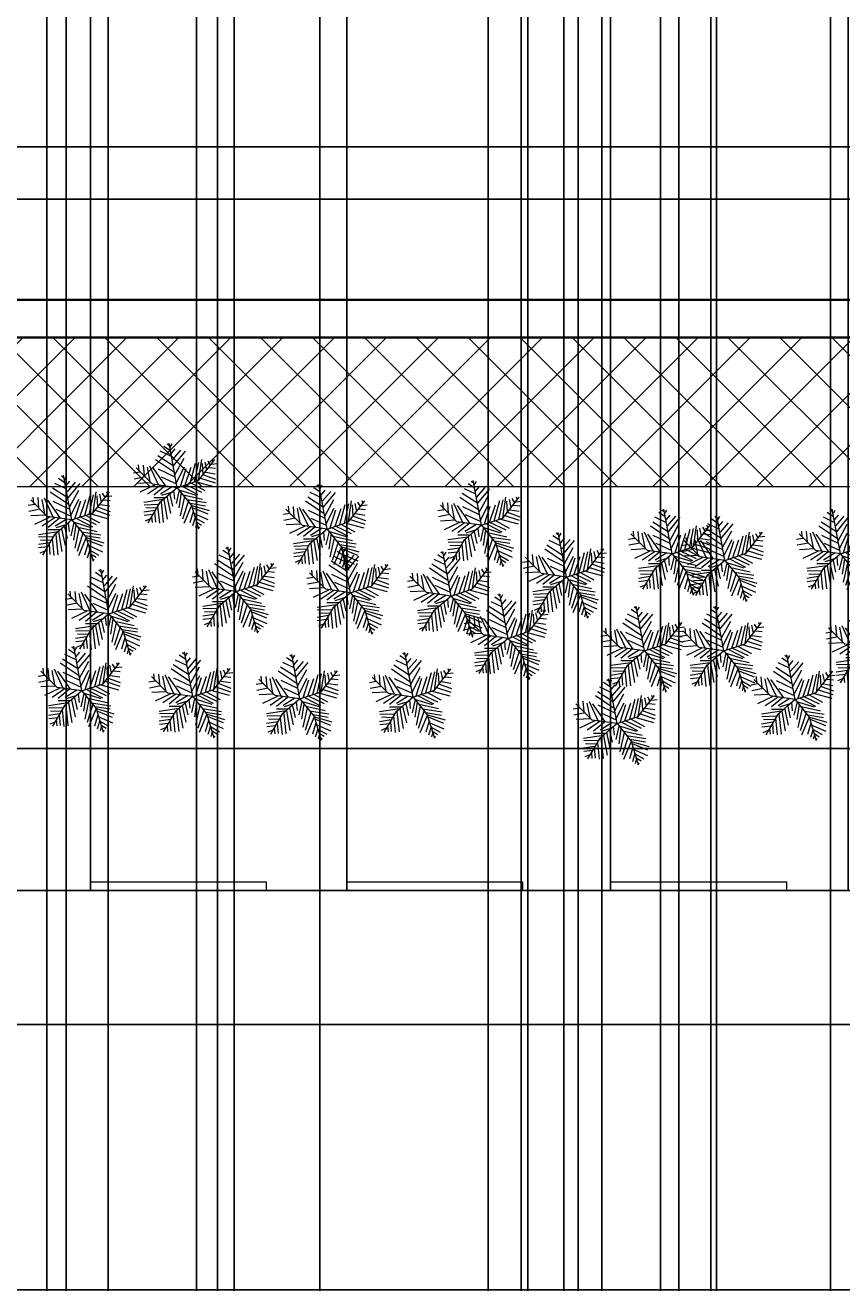
# Model space of a CAD drawing. Units: inches. Extents: x 818 to 1898, y 976 to 2364.
# Tile 17 of 96: x 1550 to 1745, y 976 to 1277. Entities that reach past the tile are written whole.
import ezdxf

# ---------------------------------------------------------------- set-up
doc = ezdxf.new("R2010")
doc.units = ezdxf.units.IN
doc.header["$LTSCALE"] = 5
doc.header["$MEASUREMENT"] = 0
for name, color, linetype, lineweight in [('A-ANNO-DIMS', 2, 'Continuous', 18), ('C-PAVE-PATT', 8, 'Continuous', 9), ('C-PROP', 7, 'Continuous', 35), ('C-ROAD', 8, 'Continuous', 25), ('C-ROAD-MRKG', 7, 'Continuous', 13), ('L-PAVE', 8, 'Continuous', 18)]:
    doc.layers.add(name, color=color, linetype=linetype, lineweight=lineweight)
doc.layers.add('L-PLNT', color=116, linetype='Continuous', lineweight=13, true_color=0x136734)
doc.styles.get("Standard").update_dxf_attribs({"font": 'arial.ttf'})
doc.dimstyles.get("Standard").update_dxf_attribs({"dimtxt": 0.18, "dimasz": 0.18, "dimexe": 0.18, "dimexo": 0.0625, "dimgap": 0.09, "dimtad": 0, "dimtih": 1, "dimtoh": 1, "dimdec": 4, "dimzin": 0, "dimdsep": 46, "dimtxsty": 'Standard', "dimcen": 0.09, "dimadec": 0, "dimazin": 0, "dimtfac": 1, "dimtdec": 4, "dimtofl": 0, "dimtmove": 0, "dimatfit": 3, "dimfxl": 1, "dimtolj": 1, "dimtzin": 0, "dimarcsym": 0})

# ---------------------------------------------------------------- blocks, each defined once
blk = doc.blocks.new('SHRUB-ACCENT')
for p, q in [((9.08, 17.24), (6.37, 18.54)), ((8.8, 18.63), (7.25, 19.67)), ((8.53, 19.84), (7.99, 20.28)), ((10.44, 9.82), (8.47, 20.47)), ((8.74, 19.5), (9.21, 20.28)), ((9.01, 17.93), (9.96, 19.06)), ((9.35, 16.54), (11.31, 18.8)), ((9.48, 14.98), (12.39, 18.54)), ((1.35, 13.77), (1.22, 15.24)), ((2.3, 15.16), (2.51, 12.72)), ((9.75, 13.42), (5.28, 16.46)), ((9.48, 15.07), (5.82, 17.41)), ((9.89, 12.9), (12.06, 16.89)), ((13.48, 10.9), (14.76, 15.68)), ((14.56, 11.16), (15.58, 15.85)), ((15.49, 11.5), (19.41, 16.55)), ((15.51, 11.51), (16.25, 16.54)), ((16.39, 15.59), (16.53, 12.9)), ((17, 15.94), (17.41, 14.03)), ((17.68, 16.2), (18.29, 15.16)), ((18.62, 15.42), (19.98, 15.59)), ((18.69, 16.63), (18.9, 15.94)), ((1.56, 13.51), (0, 13.25)), ((2.84, 12.38), (0.14, 11.86)), ((4.55, 10.66), (0.62, 14.58)), ((3.25, 14.72), (3.93, 11.25)), ((3.79, 15.07), (5.89, 10.55)), ((7.72, 10.21), (4.67, 14.55)), ((5.89, 14.29), (9.89, 12.38)), ((6.57, 12.38), (10.23, 10.73)), ((10.23, 11.07), (12.12, 14.81)), ((11.17, 10.12), (12.53, 14.37)), ((12.33, 10.47), (13.75, 14.72)), ((15.98, 12.12), (19.44, 10.99)), ((16.66, 12.9), (19.57, 11.86)), ((17.2, 13.51), (19.44, 13.16)), ((18.02, 14.63), (19.57, 14.46)), ((4.2, 10.99), (0.68, 10.81)), ((5.15, 10.47), (1.49, 8.73)), ((6.43, 10.38), (3.32, 8.3)), ((10.44, 9.82), (4.55, 10.66)), ((7.45, 10.21), (4.81, 8.04)), ((10.44, 9.82), (6.23, 6.17)), ((9.21, 10.03), (6.43, 8.3)), ((9.55, 9.16), (9.75, 7.08)), ((10.9, 9.25), (10.16, 6.04)), ((10.44, 9.82), (15.49, 11.5)), ((10.44, 9.82), (13.8, 5.61)), ((10.77, 9.34), (14.97, 8.04)), ((11.65, 10.12), (15.31, 8.21)), ((12.53, 10.47), (16.19, 8.73)), ((13.82, 10.9), (17, 9.16)), ((14.97, 11.25), (19.17, 10.12)), ((7.18, 6.99), (2.44, 6.3)), ((6.23, 6.17), (3.43, 1.4)), ((7.59, 7.43), (4.81, 7.43)), ((6.57, 6.39), (7.11, 1.52)), ((9.21, 8.73), (6.7, 7.95)), ((7.25, 6.99), (8.06, 2.31)), ((7.92, 7.69), (8.8, 3.69)), ((8.67, 8.21), (9.28, 5.43)), ((11.38, 8.64), (10.84, 5)), ((12.12, 7.69), (11.11, 3.09)), ((13.07, 6.65), (11.65, 2.31)), ((11.85, 8.12), (16.46, 7.08)), ((12.73, 6.99), (17.34, 6.3)), ((13.48, 6.13), (17.2, 5.52)), ((5.15, 4.39), (2.44, 3.95)), ((5.89, 5.78), (2.51, 5.69)), ((4.67, 3.43), (2.51, 3.17)), ((5.42, 4.91), (2.91, 5)), ((5.01, 4.04), (5.21, 1.61)), ((5.76, 5.34), (6.16, 1.35)), ((13.82, 5.6), (11.99, 1.26)), ((14.22, 4.13), (13.41, 1.44)), ((13.8, 5.61), (15.49, 0)), ((13.88, 5.6), (18.02, 4.39)), ((14.02, 5.08), (17.68, 3.61)), ((14.43, 3.69), (17.74, 2.22)), ((4, 2.39), (2.78, 1.87)), ((4.33, 2.91), (4.47, 1.52)), ((14.7, 2.74), (14.09, 0.74)), ((14.7, 2.65), (16.86, 1.44)), ((15.04, 1.26), (14.76, 0.31)), ((15.04, 1.7), (16.19, 0.92)), ((15.44, 0.48), (15.71, 0.31))]:
    blk.add_line(p, q)
blk = doc.blocks.new('LANE-STRIPE')
at = {"ltscale": 5}
for p, q in [((0, 2), (42, 2)), ((0, 2), (0, 0)), ((0, 0), (42, 0)), ((42, 2), (42, 0))]:
    blk.add_line(p, q, dxfattribs=at)
blk = doc.blocks.new('*D56')
at = {"layer": 'A-ANNO-DIMS', "color": 0, "lineweight": -2, "ltscale": 5, "transparency": 16777216}
for p, q in [((885.95, 1167.31), (885.95, 975.66)), ((1828.91, 1167.31), (1828.91, 975.66)), ((886.13, 975.84), (1357.14, 975.84)), ((1828.73, 975.84), (1357.72, 975.84))]:
    blk.add_line(p, q, dxfattribs=at)
at = {"layer": 'A-ANNO-DIMS', "color": 0, "ltscale": 5, "transparency": 16777216}
for points in [[(886.13, 975.87), (886.13, 975.81), (885.95, 975.84)], [(1828.73, 975.87), (1828.73, 975.81), (1828.91, 975.84)]]:
    blk.add_solid(points, dxfattribs=at)
at = {"layer": 'Defpoints', "color": 0, "ltscale": 5, "transparency": 16777216}
for p in [(885.95, 1167.37), (1828.91, 1167.37), (1828.91, 975.84)]:
    blk.add_point(p, dxfattribs=at)
at = {"layer": 'A-ANNO-DIMS', "color": 0, "ltscale": 5, "transparency": 16777216, "insert": (1357.43, 975.84), "char_height": 0.18, "attachment_point": 5}
blk.add_mtext('\\A1;943', dxfattribs=at)
blk = doc.blocks.new('*D58')
at = {"layer": 'A-ANNO-DIMS', "color": 0, "lineweight": -2, "ltscale": 5, "transparency": 16777216}
for p, q in [((881.51, 1159.31), (881.51, 975.66)), ((1834.44, 1145.13), (1834.44, 975.66)), ((881.69, 975.84), (1357.68, 975.84)), ((1834.26, 975.84), (1358.26, 975.84))]:
    blk.add_line(p, q, dxfattribs=at)
at = {"layer": 'A-ANNO-DIMS', "color": 0, "ltscale": 5, "transparency": 16777216}
for points in [[(881.69, 975.87), (881.69, 975.81), (881.51, 975.84)], [(1834.26, 975.87), (1834.26, 975.81), (1834.44, 975.84)]]:
    blk.add_solid(points, dxfattribs=at)
at = {"layer": 'Defpoints', "color": 0, "ltscale": 5, "transparency": 16777216}
for p in [(881.51, 1159.38), (1834.44, 1145.19), (1834.44, 975.84)]:
    blk.add_point(p, dxfattribs=at)
at = {"layer": 'A-ANNO-DIMS', "color": 0, "ltscale": 5, "transparency": 16777216, "insert": (1357.97, 975.84), "char_height": 0.18, "attachment_point": 5}
blk.add_mtext('\\A1;953', dxfattribs=at)
blk = doc.blocks.new('*D65')
at = {"layer": 'A-ANNO-DIMS', "color": 0, "lineweight": -2, "ltscale": 5, "transparency": 16777216}
for p, q in [((1430.73, 1346.02), (1430.73, 975.66)), ((1714.73, 1346.02), (1714.73, 975.66)), ((1430.91, 975.84), (1572.44, 975.84)), ((1714.55, 975.84), (1573.02, 975.84))]:
    blk.add_line(p, q, dxfattribs=at)
at = {"layer": 'A-ANNO-DIMS', "color": 0, "ltscale": 5, "transparency": 16777216}
for points in [[(1430.91, 975.87), (1430.91, 975.81), (1430.73, 975.84)], [(1714.55, 975.87), (1714.55, 975.81), (1714.73, 975.84)]]:
    blk.add_solid(points, dxfattribs=at)
at = {"layer": 'Defpoints', "color": 0, "ltscale": 5, "transparency": 16777216}
for p in [(1430.73, 1346.08), (1714.73, 1346.08), (1714.73, 975.84)]:
    blk.add_point(p, dxfattribs=at)
at = {"layer": 'A-ANNO-DIMS', "color": 0, "ltscale": 5, "transparency": 16777216, "insert": (1572.73, 975.84), "char_height": 0.18, "attachment_point": 5}
blk.add_mtext('\\A1;284', dxfattribs=at)
blk = doc.blocks.new('*D66')
at = {"layer": 'A-ANNO-DIMS', "color": 0, "lineweight": -2, "ltscale": 5, "transparency": 16777216}
for p, q in [((1714.73, 1346.02), (1714.73, 975.66)), ((1789.72, 1298.44), (1789.72, 975.66)), ((1714.91, 975.84), (1751.83, 975.84)), ((1789.54, 975.84), (1752.61, 975.84))]:
    blk.add_line(p, q, dxfattribs=at)
at = {"layer": 'A-ANNO-DIMS', "color": 0, "ltscale": 5, "transparency": 16777216}
for points in [[(1714.91, 975.87), (1714.91, 975.81), (1714.73, 975.84)], [(1789.54, 975.87), (1789.54, 975.81), (1789.72, 975.84)]]:
    blk.add_solid(points, dxfattribs=at)
at = {"layer": 'Defpoints', "color": 0, "ltscale": 5, "transparency": 16777216}
for p in [(1714.73, 1346.08), (1789.72, 1298.5), (1789.72, 975.84)]:
    blk.add_point(p, dxfattribs=at)
at = {"layer": 'A-ANNO-DIMS', "color": 0, "ltscale": 5, "transparency": 16777216, "insert": (1752.22, 975.84), "char_height": 0.18, "attachment_point": 5}
blk.add_mtext('\\A1;74.99', dxfattribs=at)
blk = doc.blocks.new('*D70')
at = {"layer": 'A-ANNO-DIMS', "color": 0, "lineweight": -2, "ltscale": 5, "transparency": 16777216}
for p, q in [((1714.79, 1346.08), (1897.92, 1346.08)), ((1897.74, 1345.9), (1897.74, 1274.7)), ((1897.74, 1203.14), (1897.74, 1274.34)), ((1798.78, 1202.96), (1897.92, 1202.96))]:
    blk.add_line(p, q, dxfattribs=at)
at = {"layer": 'A-ANNO-DIMS', "color": 0, "ltscale": 5, "transparency": 16777216}
for points in [[(1897.71, 1345.9), (1897.77, 1345.9), (1897.74, 1346.08)], [(1897.71, 1203.14), (1897.77, 1203.14), (1897.74, 1202.96)]]:
    blk.add_solid(points, dxfattribs=at)
at = {"layer": 'Defpoints', "color": 0, "ltscale": 5, "transparency": 16777216}
for p in [(1714.73, 1346.08), (1897.74, 1346.08), (1798.72, 1202.96)]:
    blk.add_point(p, dxfattribs=at)
at = {"layer": 'A-ANNO-DIMS', "color": 0, "ltscale": 5, "transparency": 16777216, "insert": (1897.74, 1274.52), "char_height": 0.18, "attachment_point": 5}
blk.add_mtext('\\A1;143.1', dxfattribs=at)
blk = doc.blocks.new('*D89')
at = {"layer": 'A-ANNO-DIMS', "color": 0, "lineweight": -2, "ltscale": 5, "transparency": 16777216}
for p, q in [((905.01, 1071.06), (1897.92, 1071.06)), ((1897.74, 1070.88), (1897.74, 1055.28)), ((1897.74, 1039.32), (1897.74, 1054.92)), ((896.18, 1039.14), (1897.92, 1039.14))]:
    blk.add_line(p, q, dxfattribs=at)
at = {"layer": 'A-ANNO-DIMS', "color": 0, "ltscale": 5, "transparency": 16777216}
for points in [[(1897.71, 1070.88), (1897.77, 1070.88), (1897.74, 1071.06)], [(1897.71, 1039.32), (1897.77, 1039.32), (1897.74, 1039.14)]]:
    blk.add_solid(points, dxfattribs=at)
at = {"layer": 'Defpoints', "color": 0, "ltscale": 5, "transparency": 16777216}
for p in [(904.95, 1071.06), (1897.74, 1071.06), (896.11, 1039.14)]:
    blk.add_point(p, dxfattribs=at)
at = {"layer": 'A-ANNO-DIMS', "color": 0, "ltscale": 5, "transparency": 16777216, "insert": (1897.74, 1055.1), "char_height": 0.18, "attachment_point": 5}
blk.add_mtext('\\A1;31.91', dxfattribs=at)
blk = doc.blocks.new('*D101')
at = {"layer": 'A-ANNO-DIMS', "color": 0, "lineweight": -2, "ltscale": 5, "transparency": 16777216}
for p, q in [((1507.3, 1071.12), (1507.3, 2363.87)), ((1507.48, 2363.69), (1536, 2363.69)), ((1565.3, 2363.69), (1536.78, 2363.69)), ((1565.48, 1071.12), (1565.48, 2363.87))]:
    blk.add_line(p, q, dxfattribs=at)
at = {"layer": 'A-ANNO-DIMS', "color": 0, "ltscale": 5, "transparency": 16777216}
for points in [[(1507.48, 2363.72), (1507.48, 2363.66), (1507.3, 2363.69)], [(1565.3, 2363.72), (1565.3, 2363.66), (1565.48, 2363.69)]]:
    blk.add_solid(points, dxfattribs=at)
at = {"layer": 'Defpoints', "color": 0, "ltscale": 5, "transparency": 16777216}
for p in [(1565.48, 2363.69), (1507.3, 1071.06), (1565.48, 1071.06)]:
    blk.add_point(p, dxfattribs=at)
at = {"layer": 'A-ANNO-DIMS', "color": 0, "ltscale": 5, "transparency": 16777216, "insert": (1536.39, 2363.69), "char_height": 0.18, "attachment_point": 5}
blk.add_mtext('\\A1;58.19', dxfattribs=at)
blk = doc.blocks.new('*D102')
at = {"layer": 'A-ANNO-DIMS', "color": 0, "lineweight": -2, "ltscale": 5, "transparency": 16777216}
for p, q in [((1565.48, 1071.12), (1565.48, 2363.87)), ((1565.66, 2363.69), (1595.63, 2363.69)), ((1626.39, 2363.69), (1596.42, 2363.69)), ((1626.57, 1071.12), (1626.57, 2363.87))]:
    blk.add_line(p, q, dxfattribs=at)
at = {"layer": 'A-ANNO-DIMS', "color": 0, "ltscale": 5, "transparency": 16777216}
for points in [[(1565.66, 2363.72), (1565.66, 2363.66), (1565.48, 2363.69)], [(1626.39, 2363.72), (1626.39, 2363.66), (1626.57, 2363.69)]]:
    blk.add_solid(points, dxfattribs=at)
at = {"layer": 'Defpoints', "color": 0, "ltscale": 5, "transparency": 16777216}
for p in [(1626.57, 2363.69), (1565.48, 1071.06), (1626.57, 1071.06)]:
    blk.add_point(p, dxfattribs=at)
at = {"layer": 'A-ANNO-DIMS', "color": 0, "ltscale": 5, "transparency": 16777216, "insert": (1596.03, 2363.69), "char_height": 0.18, "attachment_point": 5}
blk.add_mtext('\\A1;61.09', dxfattribs=at)
blk = doc.blocks.new('*D103')
at = {"layer": 'A-ANNO-DIMS', "color": 0, "lineweight": -2, "ltscale": 5, "transparency": 16777216}
for p, q in [((1626.57, 1071.12), (1626.57, 2363.87)), ((1626.75, 2363.69), (1657.7, 2363.69)), ((1689.29, 2363.69), (1658.35, 2363.69)), ((1689.47, 1071.12), (1689.47, 2363.87))]:
    blk.add_line(p, q, dxfattribs=at)
at = {"layer": 'A-ANNO-DIMS', "color": 0, "ltscale": 5, "transparency": 16777216}
for points in [[(1626.75, 2363.72), (1626.75, 2363.66), (1626.57, 2363.69)], [(1689.29, 2363.72), (1689.29, 2363.66), (1689.47, 2363.69)]]:
    blk.add_solid(points, dxfattribs=at)
at = {"layer": 'Defpoints', "color": 0, "ltscale": 5, "transparency": 16777216}
for p in [(1689.47, 2363.69), (1626.57, 1071.06), (1689.47, 1071.06)]:
    blk.add_point(p, dxfattribs=at)
at = {"layer": 'A-ANNO-DIMS', "color": 0, "ltscale": 5, "transparency": 16777216, "insert": (1658.02, 2363.69), "char_height": 0.18, "attachment_point": 5}
blk.add_mtext('\\A1;62.9', dxfattribs=at)
blk = doc.blocks.new('*D104')
at = {"layer": 'A-ANNO-DIMS', "color": 0, "lineweight": -2, "ltscale": 5, "transparency": 16777216}
for p, q in [((1689.47, 1071.12), (1689.47, 2363.87)), ((1689.65, 2363.69), (1717.4, 2363.69)), ((1745.9, 2363.69), (1718.15, 2363.69)), ((1746.08, 1071.12), (1746.08, 2363.87))]:
    blk.add_line(p, q, dxfattribs=at)
at = {"layer": 'A-ANNO-DIMS', "color": 0, "ltscale": 5, "transparency": 16777216}
for points in [[(1689.65, 2363.72), (1689.65, 2363.66), (1689.47, 2363.69)], [(1745.9, 2363.72), (1745.9, 2363.66), (1746.08, 2363.69)]]:
    blk.add_solid(points, dxfattribs=at)
at = {"layer": 'Defpoints', "color": 0, "ltscale": 5, "transparency": 16777216}
for p in [(1746.08, 2363.69), (1689.47, 1071.06), (1746.08, 1071.06)]:
    blk.add_point(p, dxfattribs=at)
at = {"layer": 'A-ANNO-DIMS', "color": 0, "ltscale": 5, "transparency": 16777216, "insert": (1717.78, 2363.69), "char_height": 0.18, "attachment_point": 5}
blk.add_mtext('\\A1;56.61', dxfattribs=at)
blk = doc.blocks.new('*D110')
at = {"layer": 'A-ANNO-DIMS', "color": 0, "lineweight": -2, "ltscale": 5, "transparency": 16777216}
for p, q in [((1164.62, 1248.46), (1897.92, 1248.46)), ((1897.74, 1248.28), (1897.74, 1242.4)), ((1897.74, 1236.14), (1897.74, 1242.03)), ((1116.25, 1235.96), (1897.92, 1235.96))]:
    blk.add_line(p, q, dxfattribs=at)
at = {"layer": 'A-ANNO-DIMS', "color": 0, "ltscale": 5, "transparency": 16777216}
for points in [[(1897.71, 1248.28), (1897.77, 1248.28), (1897.74, 1248.46)], [(1897.71, 1236.14), (1897.77, 1236.14), (1897.74, 1235.96)]]:
    blk.add_solid(points, dxfattribs=at)
at = {"layer": 'Defpoints', "color": 0, "ltscale": 5, "transparency": 16777216}
for p in [(1164.56, 1248.46), (1116.19, 1235.96), (1897.74, 1235.96)]:
    blk.add_point(p, dxfattribs=at)
at = {"layer": 'A-ANNO-DIMS', "color": 0, "ltscale": 5, "transparency": 16777216, "insert": (1897.74, 1242.21), "char_height": 0.18, "attachment_point": 5}
blk.add_mtext('\\A1;12.498', dxfattribs=at)
blk = doc.blocks.new('*D153')
at = {"layer": 'A-ANNO-DIMS', "color": 0, "lineweight": -2, "ltscale": 5, "transparency": 16777216}
for p, q in [((1713.37, 1298.02), (1713.37, 975.66)), ((1701.37, 1286.02), (1701.37, 975.66)), ((1701.55, 975.84), (1707.16, 975.84)), ((1713.19, 975.84), (1707.58, 975.84))]:
    blk.add_line(p, q, dxfattribs=at)
at = {"layer": 'A-ANNO-DIMS', "color": 0, "ltscale": 5, "transparency": 16777216}
for points in [[(1701.55, 975.87), (1701.55, 975.81), (1701.37, 975.84)], [(1713.19, 975.87), (1713.19, 975.81), (1713.37, 975.84)]]:
    blk.add_solid(points, dxfattribs=at)
at = {"layer": 'Defpoints', "color": 0, "ltscale": 5, "transparency": 16777216}
for p in [(1713.37, 1298.08), (1701.37, 1286.08), (1713.37, 975.84)]:
    blk.add_point(p, dxfattribs=at)
at = {"layer": 'A-ANNO-DIMS', "color": 0, "ltscale": 5, "transparency": 16777216, "insert": (1707.37, 975.84), "char_height": 0.18, "attachment_point": 5}
blk.add_mtext('\\A1;12', dxfattribs=at)
blk = doc.blocks.new('*D177')
at = {"layer": 'A-ANNO-DIMS', "color": 0, "lineweight": -2, "ltscale": 5, "transparency": 16777216}
for p, q in [((1559.73, 1647.52), (1559.73, 975.66)), ((1569.73, 1647.52), (1569.73, 975.66)), ((1559.91, 975.84), (1564.52, 975.84)), ((1569.55, 975.84), (1564.94, 975.84))]:
    blk.add_line(p, q, dxfattribs=at)
at = {"layer": 'A-ANNO-DIMS', "color": 0, "ltscale": 5, "transparency": 16777216}
for points in [[(1559.91, 975.87), (1559.91, 975.81), (1559.73, 975.84)], [(1569.55, 975.87), (1569.55, 975.81), (1569.73, 975.84)]]:
    blk.add_solid(points, dxfattribs=at)
at = {"layer": 'Defpoints', "color": 0, "ltscale": 5, "transparency": 16777216}
for p in [(1559.73, 1647.58), (1569.73, 1647.58), (1569.73, 975.84)]:
    blk.add_point(p, dxfattribs=at)
at = {"layer": 'A-ANNO-DIMS', "color": 0, "ltscale": 5, "transparency": 16777216, "insert": (1564.73, 975.84), "char_height": 0.18, "attachment_point": 5}
blk.add_mtext('\\A1;10', dxfattribs=at)
blk = doc.blocks.new('*D178')
at = {"layer": 'A-ANNO-DIMS', "color": 0, "lineweight": -2, "ltscale": 5, "transparency": 16777216}
for p, q in [((1669.73, 1600.02), (1669.73, 975.66)), ((1705.73, 1600.02), (1705.73, 975.66)), ((1669.91, 975.84), (1687.51, 975.84)), ((1705.55, 975.84), (1687.94, 975.84))]:
    blk.add_line(p, q, dxfattribs=at)
at = {"layer": 'A-ANNO-DIMS', "color": 0, "ltscale": 5, "transparency": 16777216}
for points in [[(1669.91, 975.87), (1669.91, 975.81), (1669.73, 975.84)], [(1705.55, 975.87), (1705.55, 975.81), (1705.73, 975.84)]]:
    blk.add_solid(points, dxfattribs=at)
at = {"layer": 'Defpoints', "color": 0, "ltscale": 5, "transparency": 16777216}
for p in [(1669.73, 1600.08), (1705.73, 1600.08), (1705.73, 975.84)]:
    blk.add_point(p, dxfattribs=at)
at = {"layer": 'A-ANNO-DIMS', "color": 0, "ltscale": 5, "transparency": 16777216, "insert": (1687.73, 975.84), "char_height": 0.18, "attachment_point": 5}
blk.add_mtext('\\A1;36', dxfattribs=at)
blk = doc.blocks.new('*D180')
at = {"layer": 'A-ANNO-DIMS', "color": 0, "lineweight": -2, "ltscale": 5, "transparency": 16777216}
for p, q in [((1599.73, 1639.52), (1599.73, 975.66)), ((1669.73, 1639.52), (1669.73, 975.66)), ((1599.91, 975.84), (1634.51, 975.84)), ((1669.55, 975.84), (1634.94, 975.84))]:
    blk.add_line(p, q, dxfattribs=at)
at = {"layer": 'A-ANNO-DIMS', "color": 0, "ltscale": 5, "transparency": 16777216}
for points in [[(1599.91, 975.87), (1599.91, 975.81), (1599.73, 975.84)], [(1669.55, 975.87), (1669.55, 975.81), (1669.73, 975.84)]]:
    blk.add_solid(points, dxfattribs=at)
at = {"layer": 'Defpoints', "color": 0, "ltscale": 5, "transparency": 16777216}
for p in [(1599.73, 1639.58), (1669.73, 1639.58), (1669.73, 975.84)]:
    blk.add_point(p, dxfattribs=at)
at = {"layer": 'A-ANNO-DIMS', "color": 0, "ltscale": 5, "transparency": 16777216, "insert": (1634.73, 975.84), "char_height": 0.18, "attachment_point": 5}
blk.add_mtext('\\A1;70', dxfattribs=at)
blk = doc.blocks.new('*D182')
at = {"layer": 'A-ANNO-DIMS', "color": 0, "lineweight": -2, "ltscale": 5, "transparency": 16777216}
for p, q in [((1463.73, 1687.02), (1463.73, 975.66)), ((1559.73, 1687.02), (1559.73, 975.66)), ((1463.91, 975.84), (1511.51, 975.84)), ((1559.55, 975.84), (1511.94, 975.84))]:
    blk.add_line(p, q, dxfattribs=at)
at = {"layer": 'A-ANNO-DIMS', "color": 0, "ltscale": 5, "transparency": 16777216}
for points in [[(1463.91, 975.87), (1463.91, 975.81), (1463.73, 975.84)], [(1559.55, 975.87), (1559.55, 975.81), (1559.73, 975.84)]]:
    blk.add_solid(points, dxfattribs=at)
at = {"layer": 'Defpoints', "color": 0, "ltscale": 5, "transparency": 16777216}
for p in [(1463.73, 1687.08), (1559.73, 1687.08), (1559.73, 975.84)]:
    blk.add_point(p, dxfattribs=at)
at = {"layer": 'A-ANNO-DIMS', "color": 0, "ltscale": 5, "transparency": 16777216, "insert": (1511.73, 975.84), "char_height": 0.18, "attachment_point": 5}
blk.add_mtext('\\A1;96', dxfattribs=at)
blk = doc.blocks.new('*D183')
at = {"layer": 'A-ANNO-DIMS', "color": 0, "lineweight": -2, "ltscale": 5, "transparency": 16777216}
for p, q in [((1714.73, 1545.02), (1714.73, 975.66)), ((1741.84, 1545.02), (1741.84, 975.66)), ((1714.91, 975.84), (1727.82, 975.84)), ((1741.66, 975.84), (1728.75, 975.84))]:
    blk.add_line(p, q, dxfattribs=at)
at = {"layer": 'A-ANNO-DIMS', "color": 0, "ltscale": 5, "transparency": 16777216}
for points in [[(1714.91, 975.87), (1714.91, 975.81), (1714.73, 975.84)], [(1741.66, 975.87), (1741.66, 975.81), (1741.84, 975.84)]]:
    blk.add_solid(points, dxfattribs=at)
at = {"layer": 'Defpoints', "color": 0, "ltscale": 5, "transparency": 16777216}
for p in [(1714.73, 1545.08), (1741.84, 1545.08), (1741.84, 975.84)]:
    blk.add_point(p, dxfattribs=at)
at = {"layer": 'A-ANNO-DIMS', "color": 0, "ltscale": 5, "transparency": 16777216, "insert": (1728.28, 975.84), "char_height": 0.18, "attachment_point": 5}
blk.add_mtext('\\A1;27.116', dxfattribs=at)
blk = doc.blocks.new('*D192')
at = {"layer": 'A-ANNO-DIMS', "color": 0, "lineweight": -2, "ltscale": 5, "transparency": 16777216}
for p, q in [((1555.13, 1338.8), (1555.13, 975.66)), ((1660.31, 1338.8), (1660.31, 975.66)), ((1555.31, 975.84), (1607.27, 975.84)), ((1660.13, 975.84), (1608.18, 975.84))]:
    blk.add_line(p, q, dxfattribs=at)
at = {"layer": 'A-ANNO-DIMS', "color": 0, "ltscale": 5, "transparency": 16777216}
for points in [[(1555.31, 975.87), (1555.31, 975.81), (1555.13, 975.84)], [(1660.13, 975.87), (1660.13, 975.81), (1660.31, 975.84)]]:
    blk.add_solid(points, dxfattribs=at)
at = {"layer": 'Defpoints', "color": 0, "ltscale": 5, "transparency": 16777216}
for p in [(1555.13, 1338.87), (1660.31, 1338.87), (1660.31, 975.84)]:
    blk.add_point(p, dxfattribs=at)
at = {"layer": 'A-ANNO-DIMS', "color": 0, "ltscale": 5, "transparency": 16777216, "insert": (1607.72, 975.84), "char_height": 0.18, "attachment_point": 5}
blk.add_mtext('\\A1;105.18', dxfattribs=at)
blk = doc.blocks.new('*D198')
at = {"layer": 'A-ANNO-DIMS', "color": 0, "lineweight": -2, "ltscale": 5, "transparency": 16777216}
for p, q in [((1741.84, 1545.02), (1741.84, 975.66)), ((1430.73, 1346.02), (1430.73, 975.66)), ((1430.91, 975.84), (1585.91, 975.84)), ((1741.66, 975.84), (1586.66, 975.84))]:
    blk.add_line(p, q, dxfattribs=at)
at = {"layer": 'A-ANNO-DIMS', "color": 0, "ltscale": 5, "transparency": 16777216}
for points in [[(1430.91, 975.87), (1430.91, 975.81), (1430.73, 975.84)], [(1741.66, 975.87), (1741.66, 975.81), (1741.84, 975.84)]]:
    blk.add_solid(points, dxfattribs=at)
at = {"layer": 'Defpoints', "color": 0, "ltscale": 5, "transparency": 16777216}
for p in [(1741.84, 1545.08), (1430.73, 1346.08), (1741.84, 975.84)]:
    blk.add_point(p, dxfattribs=at)
at = {"layer": 'A-ANNO-DIMS', "color": 0, "ltscale": 5, "transparency": 16777216, "insert": (1586.28, 975.84), "char_height": 0.18, "attachment_point": 5}
blk.add_mtext('\\A1;311.1', dxfattribs=at)
blk = doc.blocks.new('*D200')
at = {"layer": 'A-ANNO-DIMS', "color": 0, "lineweight": -2, "ltscale": 5, "transparency": 16777216}
for p, q in [((1678.33, 1477.36), (1678.33, 975.66)), ((1705.73, 1477.36), (1705.73, 975.66)), ((1678.51, 975.84), (1691.56, 975.84)), ((1705.55, 975.84), (1692.49, 975.84))]:
    blk.add_line(p, q, dxfattribs=at)
at = {"layer": 'A-ANNO-DIMS', "color": 0, "ltscale": 5, "transparency": 16777216}
for points in [[(1678.51, 975.87), (1678.51, 975.81), (1678.33, 975.84)], [(1705.55, 975.87), (1705.55, 975.81), (1705.73, 975.84)]]:
    blk.add_solid(points, dxfattribs=at)
at = {"layer": 'Defpoints', "color": 0, "ltscale": 5, "transparency": 16777216}
for p in [(1678.33, 1477.43), (1705.73, 1477.43), (1705.73, 975.84)]:
    blk.add_point(p, dxfattribs=at)
at = {"layer": 'A-ANNO-DIMS', "color": 0, "ltscale": 5, "transparency": 16777216, "insert": (1692.03, 975.84), "char_height": 0.18, "attachment_point": 5}
blk.add_mtext('\\A1;27.395', dxfattribs=at)
blk = doc.blocks.new('*D212')
at = {"layer": 'A-ANNO-DIMS', "color": 0, "lineweight": -2, "ltscale": 5, "transparency": 16777216}
for p, q in [((1681.73, 1900.02), (1681.73, 975.66)), ((1705.73, 1876.02), (1705.73, 975.66)), ((1681.91, 975.84), (1693.51, 975.84)), ((1705.55, 975.84), (1693.95, 975.84))]:
    blk.add_line(p, q, dxfattribs=at)
at = {"layer": 'A-ANNO-DIMS', "color": 0, "ltscale": 5, "transparency": 16777216}
for points in [[(1681.91, 975.87), (1681.91, 975.81), (1681.73, 975.84)], [(1705.55, 975.87), (1705.55, 975.81), (1705.73, 975.84)]]:
    blk.add_solid(points, dxfattribs=at)
at = {"layer": 'Defpoints', "color": 0, "ltscale": 5, "transparency": 16777216}
for p in [(1681.73, 1900.08), (1705.73, 1876.08), (1705.73, 975.84)]:
    blk.add_point(p, dxfattribs=at)
at = {"layer": 'A-ANNO-DIMS', "color": 0, "ltscale": 5, "transparency": 16777216, "insert": (1693.73, 975.84), "char_height": 0.18, "attachment_point": 5}
blk.add_mtext('\\A1;24', dxfattribs=at)
blk = doc.blocks.new('*D214')
at = {"layer": 'A-ANNO-DIMS', "color": 0, "lineweight": -2, "ltscale": 5, "transparency": 16777216}
for p, q in [((1511.73, 1687.02), (1511.73, 975.66)), ((1714.73, 1687.02), (1714.73, 975.66)), ((1511.91, 975.84), (1612.93, 975.84)), ((1714.55, 975.84), (1613.52, 975.84))]:
    blk.add_line(p, q, dxfattribs=at)
at = {"layer": 'A-ANNO-DIMS', "color": 0, "ltscale": 5, "transparency": 16777216}
for points in [[(1511.91, 975.87), (1511.91, 975.81), (1511.73, 975.84)], [(1714.55, 975.87), (1714.55, 975.81), (1714.73, 975.84)]]:
    blk.add_solid(points, dxfattribs=at)
at = {"layer": 'Defpoints', "color": 0, "ltscale": 5, "transparency": 16777216}
for p in [(1511.73, 1687.08), (1714.73, 1687.08), (1714.73, 975.84)]:
    blk.add_point(p, dxfattribs=at)
at = {"layer": 'A-ANNO-DIMS', "color": 0, "ltscale": 5, "transparency": 16777216, "insert": (1613.23, 975.84), "char_height": 0.18, "attachment_point": 5}
blk.add_mtext('\\A1;203', dxfattribs=at)
blk = doc.blocks.new('*D219')
at = {"layer": 'A-ANNO-DIMS', "color": 0, "lineweight": -2, "ltscale": 5, "transparency": 16777216}
for p, q in [((1595.73, 1696.02), (1595.73, 975.66)), ((1599.73, 1696.02), (1599.73, 975.66)), ((1595.91, 975.84), (1597.57, 975.84)), ((1599.55, 975.84), (1597.88, 975.84))]:
    blk.add_line(p, q, dxfattribs=at)
at = {"layer": 'A-ANNO-DIMS', "color": 0, "ltscale": 5, "transparency": 16777216}
for points in [[(1595.91, 975.87), (1595.91, 975.81), (1595.73, 975.84)], [(1599.55, 975.87), (1599.55, 975.81), (1599.73, 975.84)]]:
    blk.add_solid(points, dxfattribs=at)
at = {"layer": 'Defpoints', "color": 0, "ltscale": 5, "transparency": 16777216}
for p in [(1595.73, 1696.08), (1599.73, 1696.08), (1599.73, 975.84)]:
    blk.add_point(p, dxfattribs=at)
at = {"layer": 'A-ANNO-DIMS', "color": 0, "ltscale": 5, "transparency": 16777216, "insert": (1597.73, 975.84), "char_height": 0.18, "attachment_point": 5}
blk.add_mtext('\\A1;4', dxfattribs=at)
blk = doc.blocks.new('*D221')
at = {"layer": 'A-ANNO-DIMS', "color": 0, "lineweight": -2, "ltscale": 5, "transparency": 16777216}
for p, q in [((1668.18, 1696.02), (1668.18, 975.66)), ((1705.73, 1696.02), (1705.73, 975.66)), ((1668.36, 975.84), (1686.56, 975.84)), ((1705.55, 975.84), (1687.35, 975.84))]:
    blk.add_line(p, q, dxfattribs=at)
at = {"layer": 'A-ANNO-DIMS', "color": 0, "ltscale": 5, "transparency": 16777216}
for points in [[(1668.36, 975.87), (1668.36, 975.81), (1668.18, 975.84)], [(1705.55, 975.87), (1705.55, 975.81), (1705.73, 975.84)]]:
    blk.add_solid(points, dxfattribs=at)
at = {"layer": 'Defpoints', "color": 0, "ltscale": 5, "transparency": 16777216}
for p in [(1668.18, 1696.08), (1705.73, 1696.08), (1705.73, 975.84)]:
    blk.add_point(p, dxfattribs=at)
at = {"layer": 'A-ANNO-DIMS', "color": 0, "ltscale": 5, "transparency": 16777216, "insert": (1686.95, 975.84), "char_height": 0.18, "attachment_point": 5}
blk.add_mtext('\\A1;37.54', dxfattribs=at)
blk = doc.blocks.new('*D228')
at = {"layer": 'A-ANNO-DIMS', "color": 0, "lineweight": -2, "ltscale": 5, "transparency": 16777216}
for p, q in [((1687.39, 1802.02), (1687.39, 975.66)), ((1705.73, 1802.02), (1705.73, 975.66)), ((1687.57, 975.84), (1696.17, 975.84)), ((1705.55, 975.84), (1696.94, 975.84))]:
    blk.add_line(p, q, dxfattribs=at)
at = {"layer": 'A-ANNO-DIMS', "color": 0, "ltscale": 5, "transparency": 16777216}
for points in [[(1687.57, 975.87), (1687.57, 975.81), (1687.39, 975.84)], [(1705.55, 975.87), (1705.55, 975.81), (1705.73, 975.84)]]:
    blk.add_solid(points, dxfattribs=at)
at = {"layer": 'Defpoints', "color": 0, "ltscale": 5, "transparency": 16777216}
for p in [(1687.39, 1802.08), (1705.73, 1802.08), (1705.73, 975.84)]:
    blk.add_point(p, dxfattribs=at)
at = {"layer": 'A-ANNO-DIMS', "color": 0, "ltscale": 5, "transparency": 16777216, "insert": (1696.56, 975.84), "char_height": 0.18, "attachment_point": 5}
blk.add_mtext('\\A1;18.33', dxfattribs=at)
blk = doc.blocks.new('*D229')
at = {"layer": 'A-ANNO-DIMS', "color": 0, "lineweight": -2, "ltscale": 5, "transparency": 16777216}
for p, q in [((1599.73, 2044.02), (1599.73, 975.66)), ((1620.14, 2036.06), (1620.14, 975.66)), ((1599.91, 975.84), (1609.47, 975.84)), ((1619.96, 975.84), (1610.4, 975.84))]:
    blk.add_line(p, q, dxfattribs=at)
at = {"layer": 'A-ANNO-DIMS', "color": 0, "ltscale": 5, "transparency": 16777216}
for points in [[(1599.91, 975.87), (1599.91, 975.81), (1599.73, 975.84)], [(1619.96, 975.87), (1619.96, 975.81), (1620.14, 975.84)]]:
    blk.add_solid(points, dxfattribs=at)
at = {"layer": 'Defpoints', "color": 0, "ltscale": 5, "transparency": 16777216}
for p in [(1599.73, 2044.08), (1620.14, 2036.12), (1620.14, 975.84)]:
    blk.add_point(p, dxfattribs=at)
at = {"layer": 'A-ANNO-DIMS', "color": 0, "ltscale": 5, "transparency": 16777216, "insert": (1609.93, 975.84), "char_height": 0.18, "attachment_point": 5}
blk.add_mtext('\\A1;20.416', dxfattribs=at)
blk = doc.blocks.new('*D243')
at = {"layer": 'A-ANNO-DIMS', "color": 0, "lineweight": -2, "ltscale": 5, "transparency": 16777216}
for p, q in [((1451.77, 2020.02), (1451.77, 975.66)), ((1590.73, 2020.02), (1590.73, 975.66)), ((1451.95, 975.84), (1520.79, 975.84)), ((1590.55, 975.84), (1521.7, 975.84))]:
    blk.add_line(p, q, dxfattribs=at)
at = {"layer": 'A-ANNO-DIMS', "color": 0, "ltscale": 5, "transparency": 16777216}
for points in [[(1451.95, 975.87), (1451.95, 975.81), (1451.77, 975.84)], [(1590.55, 975.87), (1590.55, 975.81), (1590.73, 975.84)]]:
    blk.add_solid(points, dxfattribs=at)
at = {"layer": 'Defpoints', "color": 0, "ltscale": 5, "transparency": 16777216}
for p in [(1451.77, 2020.08), (1590.73, 2020.08), (1590.73, 975.84)]:
    blk.add_point(p, dxfattribs=at)
at = {"layer": 'A-ANNO-DIMS', "color": 0, "ltscale": 5, "transparency": 16777216, "insert": (1521.25, 975.84), "char_height": 0.18, "attachment_point": 5}
blk.add_mtext('\\A1;138.96', dxfattribs=at)
blk = doc.blocks.new('*D267')
at = {"layer": 'A-ANNO-DIMS', "color": 0, "lineweight": -2, "ltscale": 5, "transparency": 16777216}
for p, q in [((1714.73, 1687.02), (1714.73, 975.66)), ((1741.84, 1687.02), (1741.84, 975.66)), ((1714.91, 975.84), (1727.82, 975.84)), ((1741.66, 975.84), (1728.75, 975.84))]:
    blk.add_line(p, q, dxfattribs=at)
at = {"layer": 'A-ANNO-DIMS', "color": 0, "ltscale": 5, "transparency": 16777216}
for points in [[(1714.91, 975.87), (1714.91, 975.81), (1714.73, 975.84)], [(1741.66, 975.87), (1741.66, 975.81), (1741.84, 975.84)]]:
    blk.add_solid(points, dxfattribs=at)
at = {"layer": 'Defpoints', "color": 0, "ltscale": 5, "transparency": 16777216}
for p in [(1714.73, 1687.08), (1741.84, 1687.08), (1741.84, 975.84)]:
    blk.add_point(p, dxfattribs=at)
at = {"layer": 'A-ANNO-DIMS', "color": 0, "ltscale": 5, "transparency": 16777216, "insert": (1728.28, 975.84), "char_height": 0.18, "attachment_point": 5}
blk.add_mtext('\\A1;27.116', dxfattribs=at)

msp = doc.modelspace()

# ---------------------------------------------------------------- hatches: boundary and pattern name
at = {"layer": 'C-PAVE-PATT', "ltscale": 5}
h = msp.add_hatch(dxfattribs=at)
h.set_pattern_fill('ANSI37', color=256, scale=70)
h.paths.add_polyline_path([(1071.7252, 1202.9642), (885.9457, 1202.9642), (885.9457, 1167.3717), (1059.7252, 1167.3717, 0.41421356), (1071.7252, 1179.3717)])
h.paths.add_polyline_path([(1828.9123, 1202.9642), (1430.7251, 1202.9642), (1430.7251, 1179.3717, 0.41421356), (1442.7252, 1167.3717), (1828.9123, 1167.3717)])

# ---------------------------------------------------------------- linework, layer by layer
at = {"layer": 'C-PROP', "ltscale": 5}
for p, q in [((1789.7173, 1211.9642), (1430.7251, 1211.9642)), ((1798.7173, 1202.9642), (992.7252, 1202.9642))]:
    msp.add_line(p, q, dxfattribs=at)
at = {"layer": 'C-ROAD', "ltscale": 5}
msp.add_lwpolyline([(1828.9123, 1104.9672), (896.1138, 1104.9672), (896.1138, 1039.1433), (1828.9123, 1039.1433)], close=True, dxfattribs=at)
at = {"layer": 'L-PAVE', "ltscale": 5}
msp.add_lwpolyline([(1430.7251, 1202.9642), (1828.9123, 1202.9642), (1828.9123, 1167.3717), (1442.7252, 1167.3717, -0.41421356), (1430.7251, 1179.3717)], format="xyb", close=True, dxfattribs=at)

# ---------------------------------------------------------------- block references
at = {"layer": 'C-ROAD-MRKG', "rotation": 180}
for p in [(1607.4846, 1073.0554), (1668.5759, 1073.0554), (1731.4726, 1073.0554)]:
    msp.add_blockref('LANE-STRIPE', p, dxfattribs=at)
at = {"layer": 'L-PLNT'}
for p in [(1575.7477, 1157.3391), (1550.6355, 1149.6451), (1611.467, 1147.4817), (1648.2632, 1148.3858), (1693.6675, 1141.5583), (1733.8019, 1141.5583), (1706.2744, 1140.0159), (1668.4709, 1136.03), (1589.7959, 1132.5463), (1617.0467, 1132.2629), (1641.0246, 1131.5095), (1559.4668, 1127.2273), (1654.5969, 1121.4139), (1687.1071, 1118.4228), (1706.0166, 1118.4228), (1740.7483, 1119.194), (1553.0224, 1108.8638), (1579.4124, 1107.5244), (1604.9824, 1106.9486), (1631.9763, 1107.4007), (1722.9965, 1106.8551), (1680.5467, 1101.0712)]:
    msp.add_blockref('SHRUB-ACCENT', p, dxfattribs=at)

# ---------------------------------------------------------------- dimensions: what is measured, and where the dimension line sits
at = {"layer": 'A-ANNO-DIMS', "ltscale": 5}
for base, p1, p2, override, picture, middle in [((1565.4835, 2363.6929), (1507.2982, 1071.0552), (1565.4835, 1071.0552), {"dimdec": 2, "dimlfac": 1, "dimrnd": 0, "dimzin": 0, "dimdsep": 46, "dimlunit": 2}, '*D101', (1536.3908, 2363.6929)), ((1626.5748, 2363.6929), (1565.4835, 1071.0552), (1626.5748, 1071.0552), {"dimdec": 2, "dimlfac": 1, "dimrnd": 0, "dimzin": 0, "dimdsep": 46, "dimlunit": 2}, '*D102', (1596.0291, 2363.6929)), ((1689.4714, 2363.6929), (1626.5748, 1071.0552), (1689.4714, 1071.0552), {"dimdec": 1, "dimlfac": 1, "dimrnd": 0, "dimzin": 0, "dimdsep": 46, "dimlunit": 2}, '*D103', (1658.0231, 2363.6929)), ((1746.0831, 2363.6929), (1689.4714, 1071.0552), (1746.0831, 1071.0552), {"dimdec": 2, "dimlfac": 1, "dimrnd": 0, "dimzin": 0, "dimdsep": 46, "dimlunit": 2}, '*D104', (1717.7772, 2363.6929)), ((1620.14159, 975.84326), (1599.72515, 2044.07824), (1620.14159, 2036.1182), {"dimdec": 3, "dimlfac": 1, "dimrnd": 0, "dimzin": 0, "dimdsep": 46, "dimlunit": 2}, '*D229', (1609.93337, 975.84326)), ((1590.7251, 975.8433), (1451.7698, 2020.0782), (1590.7251, 2020.0782), {"dimdec": 2, "dimlfac": 1, "dimrnd": 0, "dimzin": 0, "dimdsep": 46, "dimlunit": 2}, '*D243', (1521.2475, 975.8433)), ((1705.7251, 975.8433), (1681.7251, 1900.0782), (1705.7251, 1876.0782), {"dimdec": 0, "dimlfac": 1, "dimrnd": 0, "dimzin": 0, "dimdsep": 46, "dimlunit": 2}, '*D212', (1693.7251, 975.8433)), ((1705.7251, 975.8433), (1687.394, 1802.0782), (1705.7251, 1802.0782), {"dimdec": 2, "dimlfac": 1, "dimrnd": 0, "dimzin": 0, "dimdsep": 46, "dimlunit": 2}, '*D228', (1696.5596, 975.8433)), ((1599.7251, 975.8433), (1595.7251, 1696.0782), (1599.7251, 1696.0782), {"dimdec": 0, "dimlfac": 1, "dimrnd": 0, "dimzin": 0, "dimdsep": 46, "dimlunit": 2}, '*D219', (1597.7251, 975.8433)), ((1705.7251, 975.8433), (1668.1841, 1696.0782), (1705.7251, 1696.0782), {"dimdec": 2, "dimlfac": 1, "dimrnd": 0, "dimzin": 0, "dimdsep": 46, "dimlunit": 2}, '*D221', (1686.9546, 975.8433)), ((1559.7251, 975.8433), (1463.7251, 1687.0782), (1559.7251, 1687.0782), {"dimdec": 0, "dimlfac": 1, "dimrnd": 0, "dimzin": 0, "dimdsep": 46, "dimlunit": 2}, '*D182', (1511.7251, 975.8433)), ((1714.7251, 975.8433), (1511.7251, 1687.0782), (1714.7251, 1687.0782), {"dimdec": 0, "dimlfac": 1, "dimrnd": 0, "dimzin": 0, "dimdsep": 46, "dimlunit": 2}, '*D214', (1613.2251, 975.8433)), ((1741.8409, 975.8433), (1714.7251, 1687.0782), (1741.8409, 1687.0782), {"dimdec": 3, "dimlfac": 1, "dimrnd": 0, "dimzin": 0, "dimdsep": 46, "dimlunit": 2}, '*D267', (1728.283, 975.8433)), ((1569.7251, 975.8433), (1559.7251, 1647.5782), (1569.7251, 1647.5782), {"dimdec": 0, "dimlfac": 1, "dimrnd": 0, "dimzin": 0, "dimdsep": 46, "dimlunit": 2}, '*D177', (1564.7251, 975.8433)), ((1669.7251, 975.8433), (1599.7251, 1639.5782), (1669.7251, 1639.5782), {"dimdec": 0, "dimlfac": 1, "dimrnd": 0, "dimzin": 0, "dimdsep": 46, "dimlunit": 2}, '*D180', (1634.7251, 975.8433)), ((1705.7251, 975.8433), (1669.7251, 1600.0782), (1705.7251, 1600.0782), {"dimdec": 0, "dimlfac": 1, "dimrnd": 0, "dimzin": 0, "dimdsep": 46, "dimlunit": 2}, '*D178', (1687.7251, 975.8433)), ((1741.8409, 975.8433), (1430.7251, 1346.0782), (1741.8409, 1545.0782), {"dimdec": 1, "dimlfac": 1, "dimrnd": 0, "dimzin": 0, "dimdsep": 46, "dimlunit": 2}, '*D198', (1586.283, 975.8433)), ((1741.8409, 975.8433), (1714.7251, 1545.0782), (1741.8409, 1545.0782), {"dimdec": 3, "dimlfac": 1, "dimrnd": 0, "dimzin": 0, "dimdsep": 46, "dimlunit": 2}, '*D183', (1728.283, 975.8433)), ((1705.7251, 975.8433), (1678.3302, 1477.4261), (1705.7251, 1477.4261), {"dimdec": 3, "dimlfac": 1, "dimrnd": 0, "dimzin": 0, "dimdsep": 46, "dimlunit": 2}, '*D200', (1692.0277, 975.8433)), ((1714.7251, 975.8433), (1430.7251, 1346.0782), (1714.7251, 1346.0782), {"dimdec": 0, "dimlfac": 1, "dimrnd": 0, "dimzin": 0, "dimdsep": 46, "dimlunit": 2}, '*D65', (1572.7251, 975.8433)), ((1789.7173, 975.8433), (1714.7251, 1346.0782), (1789.7173, 1298.5041), {"dimdec": 2, "dimlfac": 1, "dimrnd": 0, "dimzin": 0, "dimdsep": 46, "dimlunit": 2}, '*D66', (1752.2212, 975.8433)), ((1660.3141, 975.8433), (1555.1299, 1338.8654), (1660.3141, 1338.8654), {"dimdec": 2, "dimlfac": 1, "dimrnd": 0, "dimzin": 0, "dimdsep": 46, "dimlunit": 2}, '*D192', (1607.722, 975.8433)), ((1713.3688, 975.8433), (1701.3688, 1286.0782), (1713.3688, 1298.0782), {"dimdec": 0, "dimlfac": 1, "dimrnd": 0, "dimzin": 0, "dimdsep": 46, "dimlunit": 2}, '*D153', (1707.3688, 975.8433)), ((1828.9123, 975.8433), (885.9457, 1167.3717), (1828.9123, 1167.3717), {"dimdec": 0, "dimlfac": 1, "dimrnd": 0, "dimzin": 0, "dimdsep": 46, "dimlunit": 2}, '*D56', (1357.429, 975.8433)), ((1834.436, 975.8433), (881.5059, 1159.375), (1834.436, 1145.1942), {"dimdec": 0, "dimlfac": 1, "dimrnd": 0, "dimzin": 0, "dimdsep": 46, "dimlunit": 2}, '*D58', (1357.971, 975.8433))]:
    dim = msp.add_linear_dim(base=base, p1=p1, p2=p2, dimstyle='Standard', override=override, dxfattribs=at)
    dim.commit()
    dim.dimension.update_dxf_attribs({"geometry": picture, "text_midpoint": middle})
for base, p1, p2, override, picture, middle in [((1897.736, 1346.0782), (1798.7173, 1202.9642), (1714.7251, 1346.0782), {"dimdec": 1, "dimlfac": 1, "dimrnd": 0, "dimzin": 0, "dimdsep": 46, "dimlunit": 2}, '*D70', (1897.736, 1274.5212)), ((1897.736, 1235.9642), (1164.5571, 1248.4622), (1116.1882, 1235.9642), {"dimdec": 3, "dimlfac": 1, "dimrnd": 0, "dimzin": 0, "dimdsep": 46, "dimlunit": 2}, '*D110', (1897.736, 1242.2132)), ((1897.736, 1071.0552), (896.1138, 1039.1433), (904.9504, 1071.0552), {"dimdec": 2, "dimlfac": 1, "dimrnd": 0, "dimzin": 0, "dimdsep": 46, "dimlunit": 2}, '*D89', (1897.736, 1055.0992))]:
    dim = msp.add_linear_dim(base=base, p1=p1, p2=p2, angle=90, dimstyle='Standard', override=override, dxfattribs=at)
    dim.commit()
    dim.dimension.update_dxf_attribs({"geometry": picture, "text_midpoint": middle})

doc.saveas('drawing.dxf')
